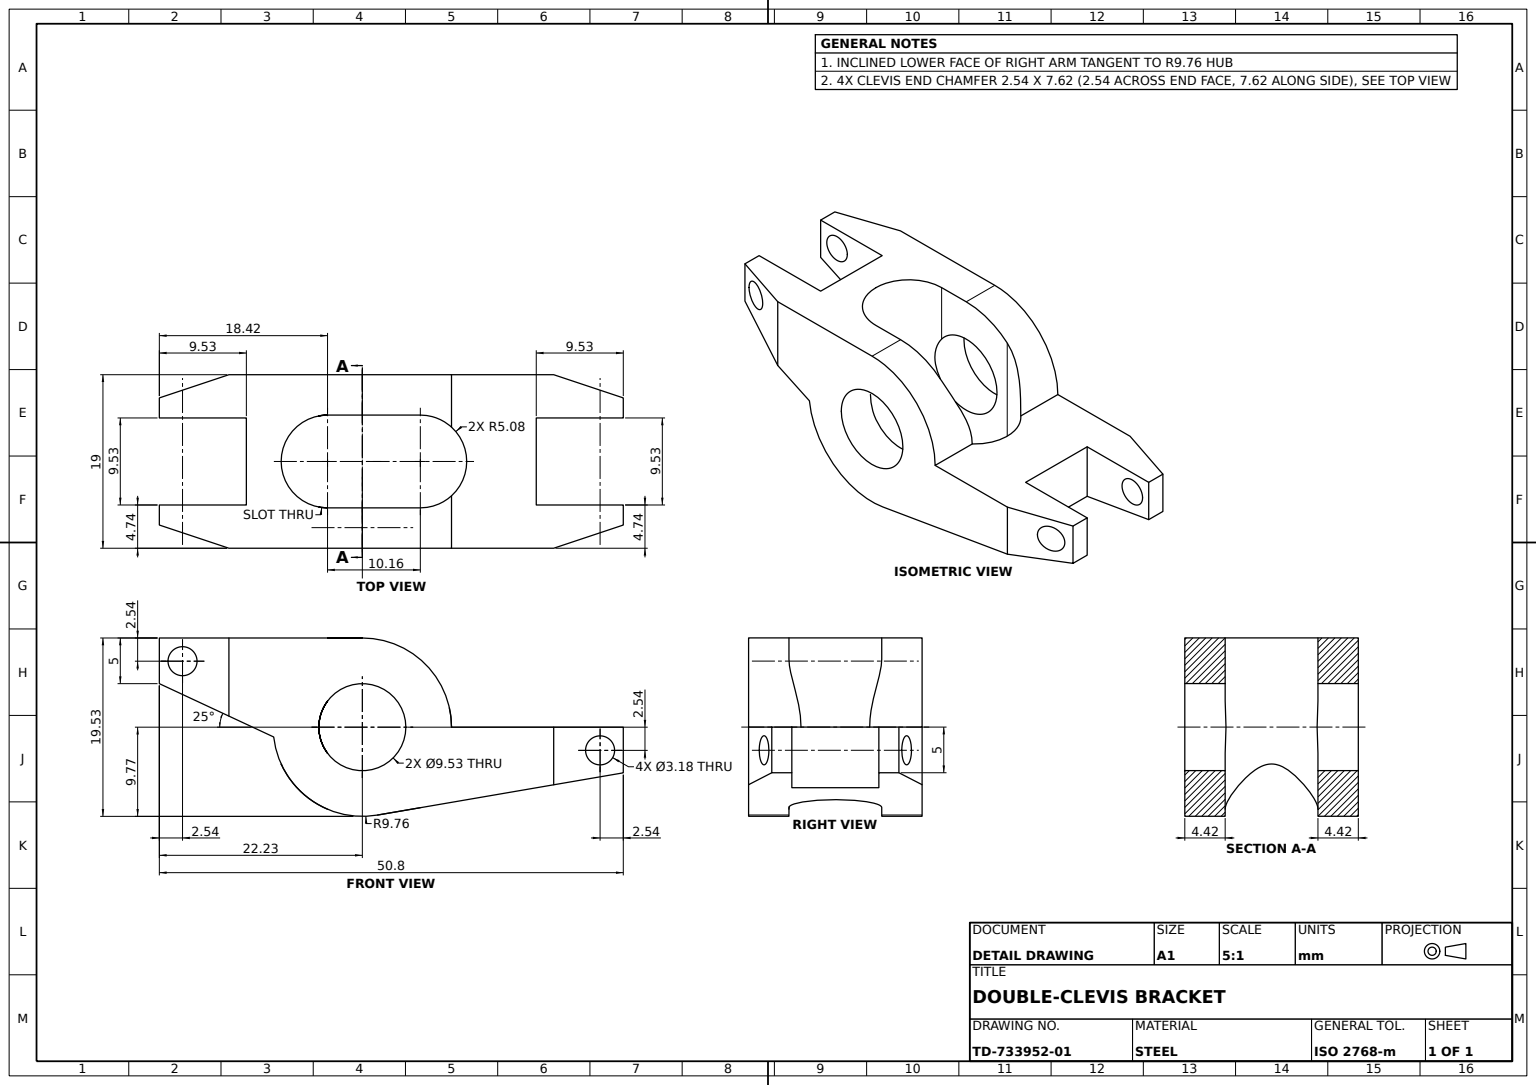
from build123d import *
from OCP.BRepFilletAPI import BRepFilletAPI_MakeChamfer

# Parameters (mm, degrees)
ROCKER_ARM_PROFILE_SKETCH_R  = 4.765
ROCKER_ARM_BODY_DEPTH        = 9.5
END_CHAMFER_2_54X7_62_SIZE   = 2.54
END_CHAMFER_2_54X7_62_SIZE2  = 7.62
END_CHAMFER_7_62X2_54_SIZE   = 7.62
END_CHAMFER_7_62X2_54_SIZE2  = 2.54
HUB_CUT_DEPTH                = 32.656529342
HUB_CUT_DEPTH_BACK           = 32.656529342
FORK_SLOT_CUT_DEPTH          = 32.656529403
FORK_SLOT_CUT_DEPTH_BACK     = 32.656529403
FORK_SLOT_SKETCH_W           = 9.53
FORK_SLOT_SKETCH_H           = 9.53
PIN_HOLES_2X_3_18_DEPTH      = 32.656529403
PIN_HOLES_2X_3_18_DEPTH_BACK = 32.656529403
PIN_HOLES_SKETCH_R           = 1.59


with BuildPart() as part:
    # Rocker Arm Profile Sketch → Rocker Arm Body (new, symmetric)
    with BuildSketch(Plane(origin=(0, 0, 0), x_dir=(0, 0, -1), z_dir=(1, 0, 0))):
        with BuildLine():
            ThreePointArc((9.765, 0), (6.904897718, 6.904897718), (0, 9.765))
            Line((0, 9.765), (-22.23, 9.765))
            Line((-22.23, 9.765), (-22.23, 4.765))
            Line((-22.23, 4.765), (-9.705624325, -1.075212291))
            ThreePointArc((-9.705624325, -1.075212291), (-5.872128035, -7.802136716), (1.653013564, -9.624072483))
            Line((1.653013564, -9.624072483), (28.575, -5))
            Line((28.575, -5), (28.575, 0))
            Line((28.575, 0), (9.765, 0))
        make_face()
        Circle(ROCKER_ARM_PROFILE_SKETCH_R, mode=Mode.SUBTRACT)
    extrude(amount=ROCKER_ARM_BODY_DEPTH, both=True)

    # End Chamfer 2.54x7.62: one chamfer whose edges measure the first distance from different faces: ONE call of the kernel's chamfer builder (chamfer() names one face for all edges)
    end_chamfer_2_54x7_62_edges_1 = [part.edges().sort_by_distance(p)[0] for p in [
        (-9.5, -2.5, -28.575),
    ]]
    end_chamfer_2_54x7_62_side_1 = [part.faces().sort_by_distance(p)[0] for p in [
        (0, -2.5, -28.575),
    ]]
    end_chamfer_2_54x7_62_edges_2 = [part.edges().sort_by_distance(p)[0] for p in [
        (9.5, 7.265, 22.23),
    ]]
    end_chamfer_2_54x7_62_side_2 = [part.faces().sort_by_distance(p)[0] for p in [
        (0, 7.265, 22.23),
    ]]
    end_chamfer_2_54x7_62 = BRepFilletAPI_MakeChamfer(part.part.solid().wrapped)
    for e in end_chamfer_2_54x7_62_edges_1:
        end_chamfer_2_54x7_62.Add(END_CHAMFER_2_54X7_62_SIZE, END_CHAMFER_2_54X7_62_SIZE2, e.wrapped, end_chamfer_2_54x7_62_side_1[0].wrapped)  # the first distance lies on this face
    for e in end_chamfer_2_54x7_62_edges_2:
        end_chamfer_2_54x7_62.Add(END_CHAMFER_2_54X7_62_SIZE, END_CHAMFER_2_54X7_62_SIZE2, e.wrapped, end_chamfer_2_54x7_62_side_2[0].wrapped)  # the first distance lies on this face
    add(Compound.cast(end_chamfer_2_54x7_62.Shape()), mode=Mode.REPLACE)

    # End Chamfer 7.62x2.54: one chamfer whose edges measure the first distance from different faces: ONE call of the kernel's chamfer builder (chamfer() names one face for all edges)
    end_chamfer_7_62x2_54_edges_1 = [part.edges().sort_by_distance(p)[0] for p in [
        (-9.5, 7.265, 22.23),
    ]]
    end_chamfer_7_62x2_54_side_1 = [part.faces().sort_by_distance(p)[0] for p in [
        (-9.5, -0.473958345, -15.36),
    ]]
    end_chamfer_7_62x2_54_edges_2 = [part.edges().sort_by_distance(p)[0] for p in [
        (9.5, -2.5, -28.575),
    ]]
    end_chamfer_7_62x2_54_side_2 = [part.faces().sort_by_distance(p)[0] for p in [
        (9.5, 9.291041655, 7.305),
    ]]
    end_chamfer_7_62x2_54 = BRepFilletAPI_MakeChamfer(part.part.solid().wrapped)
    for e in end_chamfer_7_62x2_54_edges_1:
        end_chamfer_7_62x2_54.Add(END_CHAMFER_7_62X2_54_SIZE, END_CHAMFER_7_62X2_54_SIZE2, e.wrapped, end_chamfer_7_62x2_54_side_1[0].wrapped)  # the first distance lies on this face
    for e in end_chamfer_7_62x2_54_edges_2:
        end_chamfer_7_62x2_54.Add(END_CHAMFER_7_62X2_54_SIZE, END_CHAMFER_7_62X2_54_SIZE2, e.wrapped, end_chamfer_7_62x2_54_side_2[0].wrapped)  # the first distance lies on this face
    add(Compound.cast(end_chamfer_7_62x2_54.Shape()), mode=Mode.REPLACE)

    # Hub Cut Sketch → Hub Cut (cut, two sides: drawn at the far end of the back side and taken through both)
    with BuildSketch(Plane(origin=(0, 0, 0), x_dir=(1, 0, 0), z_dir=(0, 1, 0)).offset(-HUB_CUT_DEPTH_BACK)):
        with BuildLine():
            Line((-5.08, -3.81), (-5.08, 6.35))
            ThreePointArc((-5.08, 6.35), (0, 11.43), (5.08, 6.35))
            Line((5.08, 6.35), (5.08, -3.81))
            ThreePointArc((5.08, -3.81), (0, -8.89), (-5.08, -3.81))
        make_face()
    extrude(amount=HUB_CUT_DEPTH + HUB_CUT_DEPTH_BACK, mode=Mode.SUBTRACT)

    # Fork Slot Sketch → Fork Slot Cut (cut, two sides: drawn at the far end of the back side and taken through both)
    with BuildSketch(Plane(origin=(0, 0, 0), x_dir=(1, 0, 0), z_dir=(0, 1, 0)).offset(-FORK_SLOT_CUT_DEPTH_BACK)):
        with Locations((0, 23.81)):
            Rectangle(FORK_SLOT_SKETCH_W, FORK_SLOT_SKETCH_H)
        with Locations((0, -17.465)):
            Rectangle(FORK_SLOT_SKETCH_W, FORK_SLOT_SKETCH_H)
    extrude(amount=FORK_SLOT_CUT_DEPTH + FORK_SLOT_CUT_DEPTH_BACK, mode=Mode.SUBTRACT)

    # Pin Holes Sketch → Pin Holes 2xØ3.18 (cut, two sides: drawn at the far end of the back side and taken through both)
    with BuildSketch(Plane(origin=(0, 0, 0), x_dir=(0, 0, -1), z_dir=(1, 0, 0)).offset(-PIN_HOLES_2X_3_18_DEPTH_BACK)):
        with Locations(Location((-19.69, 7.225, 0), (0, 0, 180))):
            Circle(PIN_HOLES_SKETCH_R)
        with Locations((26.035, -2.54)):
            Circle(PIN_HOLES_SKETCH_R)
    extrude(amount=PIN_HOLES_2X_3_18_DEPTH + PIN_HOLES_2X_3_18_DEPTH_BACK, mode=Mode.SUBTRACT)


solid = part.part
